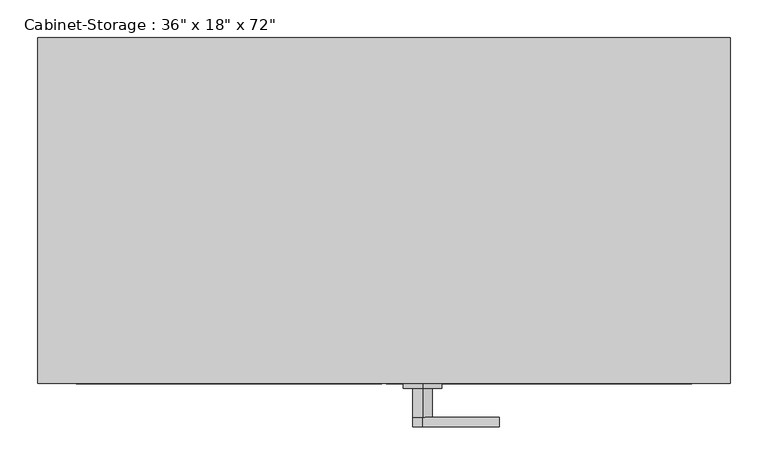
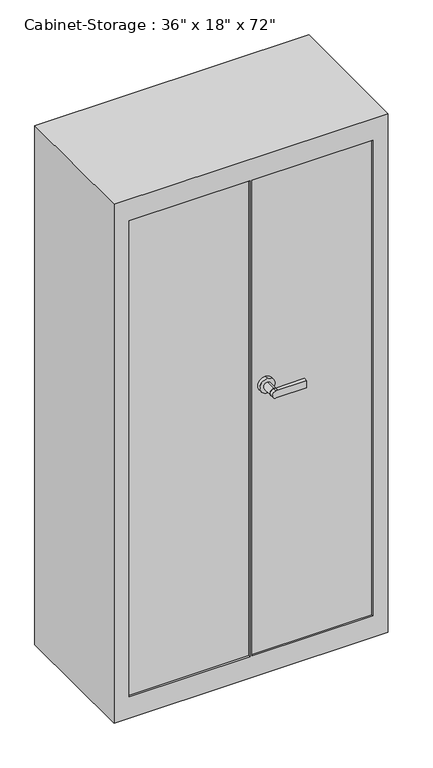
"""IFC4 building model written with IfcOpenShell, lengths in millimetres: furniture geometry."""

from ifc_helpers import new_model, si_unit, point, frame, frame_2d, origin, place, context, project, spatial, polyline, circle_curve, trimmed, segment, composite_curve, outline, extrude, faceted_brep, source, transform, mapped, element, save


def furniture_d3d70ab1(model_context):
    return source(origin(), model_context, "Body", "SolidModel", [
        faceted_brep([(457.2, -228.6, 1828.8), (457.2, 228.6, 1828.8), (-457.2, 228.6, 1828.8), (-457.2, -228.6, 1828.8), (457.2, -228.6, 0.0), (-457.2, -228.6, 0.0), (-457.2, 228.6, 0.0), (457.2, 228.6, 0.0), (406.4, -228.6, 1752.6), (406.4, -228.6, 76.2), (3.175, -228.6, 76.2), (3.175, -228.6, 1752.6), (-406.4, -228.6, 1752.6), (-3.175, -228.6, 1752.6), (-3.175, -228.6, 76.2), (-406.4, -228.6, 76.2), (406.4, -222.25, 76.2), (406.4, -222.25, 1752.6), (3.175, -222.25, 1752.6), (3.175, -222.25, 76.2), (-3.175, -222.25, 1752.6), (-406.4, -222.25, 1752.6), (-406.4, -222.25, 76.2), (-3.175, -222.25, 76.2)], [[[0, 1, 2, 3]], [[4, 5, 6, 7]], [[1, 0, 4, 7]], [[2, 1, 7, 6]], [[3, 2, 6, 5]], [[0, 3, 5, 4], [8, 9, 10, 11], [12, 13, 14, 15]], [[16, 17, 18, 19]], [[17, 16, 9, 8]], [[18, 17, 8, 11]], [[19, 18, 11, 10]], [[16, 19, 10, 9]], [[20, 21, 22, 23]], [[21, 20, 13, 12]], [[22, 21, 12, 15]], [[23, 22, 15, 14]], [[20, 23, 14, 13]]]),
        extrude(outline(composite_curve([segment(trimmed(circle_curve(frame_2d((1016.0, 50.9427411)), 25.4), [point((1041.4, 50.9427411))], [point((990.6, 50.9427411))], False, "CARTESIAN"), True, "CONTINUOUS"), segment(trimmed(circle_curve(frame_2d((1016.0, 50.9427411)), 25.4), [point((990.6, 50.9427411))], [point((1041.4, 50.9427411))], False, "CARTESIAN"), True, "CONTINUOUS")], self_intersect=False)), frame((0.0, -234.95, 0.0), z_axis=(0.0, 1.0, 0.0), x_axis=(0.0, 0.0, 1.0)), (0.0, 0.0, 1.0), 12.7),
        extrude(outline(composite_curve([segment(trimmed(circle_curve(frame_2d((1016.0, 50.9427411)), 12.7), [point((1028.7, 50.9427411))], [point((1003.3, 50.9427411))], False, "CARTESIAN"), True, "CONTINUOUS"), segment(trimmed(circle_curve(frame_2d((1016.0, 50.9427411)), 12.7), [point((1003.3, 50.9427411))], [point((1028.7, 50.9427411))], False, "CARTESIAN"), True, "CONTINUOUS")], self_intersect=False)), frame((0.0, -273.05, 0.0), z_axis=(0.0, 1.0, 0.0), x_axis=(0.0, 0.0, 1.0)), (0.0, 0.0, 1.0), 38.1),
        extrude(outline(composite_curve([segment(polyline([(1028.7, 152.5427411), (1028.7, 50.9427411)]), True, "CONTINUOUS"), segment(trimmed(circle_curve(frame_2d((1016.0, 50.9427411)), 12.7), [point((1028.7, 50.9427411))], [point((1003.3, 50.9427411))], False, "CARTESIAN"), True, "CONTINUOUS"), segment(polyline([(1003.3, 50.9427411), (1003.3, 152.5427411), (1028.7, 152.5427411)]), True, "CONTINUOUS")], self_intersect=False)), frame((0.0, -285.75, 0.0), z_axis=(0.0, 1.0, 0.0), x_axis=(0.0, 0.0, 1.0)), (0.0, 0.0, 1.0), 12.7),
    ])


if __name__ == "__main__":
    model = new_model("IFC4")
    model_context = context("Model", 3, world=origin())
    ifc_project = project(units=[si_unit("LENGTHUNIT", "METRE", prefix="MILLI")], contexts=[model_context])
    site = spatial("IfcSite", under=ifc_project)
    building = spatial("IfcBuilding", under=site)
    placement = place(None, origin())
    furniture_shape = furniture_d3d70ab1(model_context)
    element("IfcFurniture", 1, ObjectType="Cabinet-Storage : 36\" x 18\" x 72\"", at=placement, inside=building, context=model_context, shape_type="MappedRepresentation", body=[
        mapped(furniture_shape, transform((0.0, 0.0, 0.0), x_axis=(1.0, 0.0, 0.0), y_axis=(0.0, 1.0, 0.0), z_axis=(0.0, 0.0, 1.0))),
    ])
    save(model, "model.ifc")

# Revit data of these elements
# Type "Cabinet-Storage : 36\" x 18\" x 72\""
#   Assembly Code = "E2020200"
#   Depth = 1' - 6"
#   Height = 6' - 0"
#   Width = 3' - 0"
#   Material = Metal - Steel
#   Default Elevation = 0
# Element 1 (IfcFurniture, "Cabinet-Storage : 36\" x 18\" x 72\"")
#   Materials on its faces: "Metal - Steel", "Metal - Chrome"
# Materials
#   "Metal - Steel": colour RGB 247 247 247, transparency 0
#   "Metal - Chrome": colour RGB 17 17 17, transparency 0
